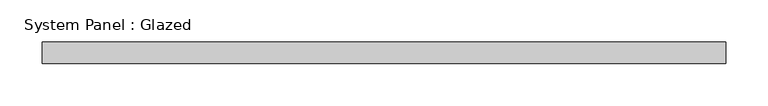
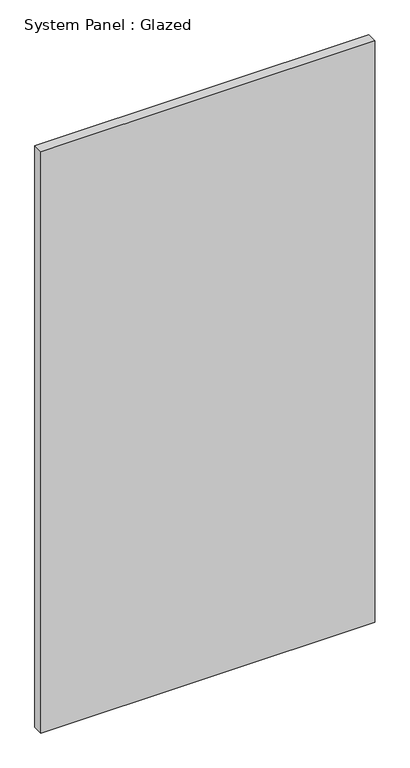
"""IFC4 building model written with IfcOpenShell, lengths in millimetres: plate geometry, System Panel : Glazed."""

from ifc_helpers import new_model, si_unit, origin, origin_with_axes, place, context, project, spatial, polyline, outline, extrude, source, transform, mapped, element, save


def system_panel_glazed_acb18a83(model_context):
    return source(origin(), model_context, "Body", "SweptSolid", [
        extrude(outline(polyline([(403.225, 19.05), (-403.225, 19.05), (-403.225, 44.45), (403.225, 44.45), (403.225, 19.05)])), origin_with_axes(), (0.0, 0.0, 1.0), 1484.7177577),
    ])


if __name__ == "__main__":
    model = new_model("IFC4")
    model_context = context("Model", 3, world=origin())
    ifc_project = project(units=[si_unit("LENGTHUNIT", "METRE", prefix="MILLI")], contexts=[model_context])
    site = spatial("IfcSite", under=ifc_project)
    building = spatial("IfcBuilding", under=site)
    placement = place(None, origin())
    system_panel_glazed_shape = system_panel_glazed_acb18a83(model_context)
    element("IfcPlate", 1, ObjectType="System Panel : Glazed", at=placement, inside=building, context=model_context, shape_type="MappedRepresentation", body=[
        mapped(system_panel_glazed_shape, transform((0.0, 0.0, 0.0), x_axis=(1.0, 0.0, 0.0), y_axis=(0.0, 1.0, 0.0), z_axis=(0.0, 0.0, 1.0))),
    ])
    save(model, "model.ifc")

# Revit data of these elements
# Type "System Panel : Glazed"
#   Construction Type Id = "GSP4R"
#   Analytic Construction = "1/8 in Pilkington single glazing"
#   Visual Light Transmittance = 0.9
#   Solar Heat Gain Coefficient = 0.86
#   Heat Transfer Coefficient (U) = 1.18115 BTU/(h·ft²·°F)
#   Define Thermal Properties by = 1
# Element 1 (IfcPlate, "System Panel : Glazed")
#   Materials on its faces: "Glass"
# Materials
#   "Glass": class "Glass", colour RGB 0 128 192, transparency 0.75, Description = "Soda Lime Glass", Cost = 0
